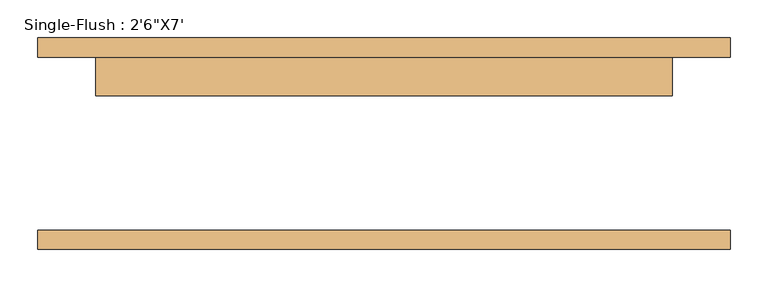
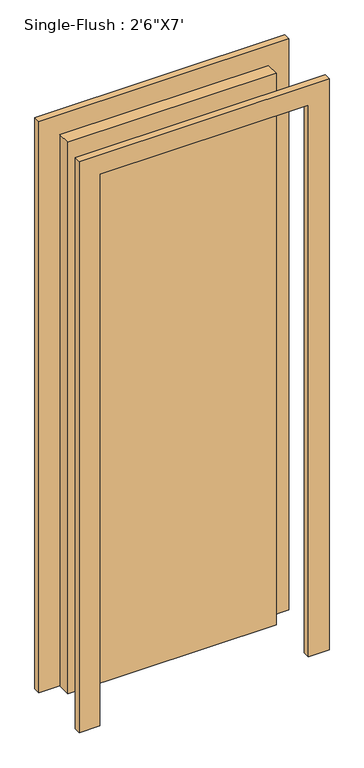
"""IFC4 building model written with IfcOpenShell, lengths in millimetres: door geometry."""

from ifc_helpers import new_model, si_unit, frame, origin, origin_with_axes, place, context, project, spatial, polyline, outline, extrude, source, transform, mapped, element, save


def door_bb98abfd(model_context):
    return source(origin(), model_context, "Body", "SweptSolid", [
        extrude(outline(polyline([(2209.8, -457.2), (0.0, -457.2), (0.0, -381.0), (2133.6, -381.0), (2133.6, 381.0), (0.0, 381.0), (0.0, 457.2), (2209.8, 457.2), (2209.8, -457.2)])), frame((0.0, 114.3, 0.0), z_axis=(0.0, 1.0, 0.0), x_axis=(0.0, 0.0, 1.0)), (0.0, 0.0, 1.0), 25.4),
        extrude(outline(polyline([(2209.8, 457.2), (2209.8, -457.2), (0.0, -457.2), (0.0, -381.0), (2133.6, -381.0), (2133.6, 381.0), (0.0, 381.0), (0.0, 457.2), (2209.8, 457.2)])), frame((0.0, -139.7, 0.0), z_axis=(0.0, 1.0, 0.0), x_axis=(0.0, 0.0, 1.0)), (0.0, 0.0, 1.0), 25.4),
        extrude(outline(polyline([(381.0, 63.5), (-381.0, 63.5), (-381.0, 114.3), (381.0, 114.3), (381.0, 63.5)])), origin_with_axes(), (0.0, 0.0, 1.0), 2133.6),
    ])


if __name__ == "__main__":
    model = new_model("IFC4")
    model_context = context("Model", 3, world=origin())
    ifc_project = project(units=[si_unit("LENGTHUNIT", "METRE", prefix="MILLI")], contexts=[model_context])
    site = spatial("IfcSite", under=ifc_project)
    building = spatial("IfcBuilding", under=site)
    placement = place(None, origin())
    door_shape = door_bb98abfd(model_context)
    element("IfcDoor", 1, ObjectType="Single-Flush : 2'6\"X7'", at=placement, inside=building, context=model_context, shape_type="MappedRepresentation", body=[
        mapped(door_shape, transform((0.0, 0.0, 0.0), x_axis=(1.0, 0.0, 0.0), y_axis=(0.0, 1.0, 0.0), z_axis=(0.0, 0.0, 1.0))),
    ])
    save(model, "model.ifc")

# Revit data of these elements
# Type "Single-Flush : 2'6\"X7'"
#   Type Mark = "10"
#   Construction Type Id = "MDOOR"
#   Assembly Code = "C1020"
#   Analytic Construction = "Metal"
#   Thickness = 0' - 2"
#   Heat Transfer Coefficient (U) = 0.651978 BTU/(h·ft²·°F)
#   Height = 7' - 0"
#   Trim Projection Ext = 0' - 1"
#   Trim Projection Int = 0' - 1"
#   Trim Width = 0' - 3"
#   Width = 2' - 6"
#   Define Thermal Properties by = 1
#   Door Material = Door - Panel
#   Frame Material = Door - Frame
#   Visual Light Transmittance = 0
#   Solar Heat Gain Coefficient = 0
#   Function = (empty or 0)
#   Wall Closure = (empty or 0)
# Element 1 (IfcDoor, "Single-Flush : 2'6\"X7'")
#   Materials on its faces: "Door - Frame", "Door - Panel"
# Materials
#   "Door - Panel": class "Wood", colour RGB 210 159 95, transparency 0, Cost = 0
#   "Door - Frame": colour RGB 118 70 51, transparency 0, Cost = 0
